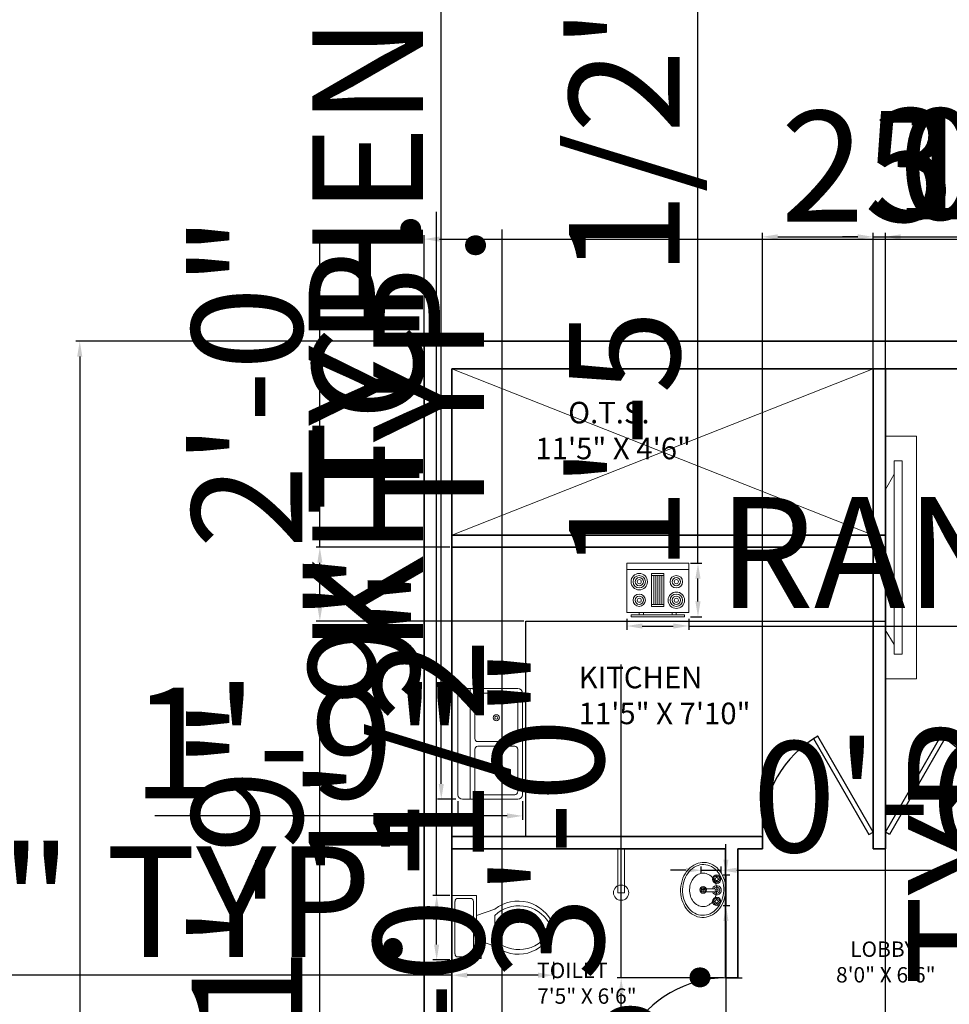
# Model space of a CAD drawing. Units: inches. Extents: x 2901 to 21549, y 2042 to 3828.
# Tile 4 of 10: x 3202 to 3505, y 3259 to 3579. Entities that reach past the tile are written whole.
import ezdxf

# ---------------------------------------------------------------- set-up
doc = ezdxf.new("R2010")
doc.units = ezdxf.units.IN
doc.layers.get('Defpoints').update_dxf_attribs({"color": 1})
for name, color, linetype, lineweight in [('A-ANNO-DIMS', 2, 'Continuous', 18), ('A-AREA-IDEN', 7, 'Continuous', 18), ('A-DOOR', 3, 'Continuous', 25), ('A-EQPM', 8, 'Continuous', 18), ('A-FLOR-CASE', 8, 'Continuous', 25), ('A-FLOR-FIXT', 9, 'Continuous', 18), ('A-ROOF-OPEN', 8, 'Continuous', 13), ('A-WALL', 7, 'Continuous', 35)]:
    doc.layers.add(name, color=color, linetype=linetype, lineweight=lineweight)
doc.styles.get("Standard").update_dxf_attribs({"font": 'arial.ttf'})
doc.dimstyles.new('ISO-25', dxfattribs={"dimtxt": 36, "dimasz": 5, "dimexe": 1.25, "dimexo": 0.625, "dimtad": 1, "dimdec": 0, "dimlunit": 3, "dimtxsty": 'Standard', "dimcen": 2.5, "dimadec": 0, "dimazin": 0, "dimtfac": 1, "dimtdec": 0, "dimtmove": 0, "dimatfit": 3, "dimfxl": 1, "dimarcsym": 0})

# ---------------------------------------------------------------- blocks, each defined once
blk = doc.blocks.new('*U21')
for p, q in [((0, 0), (0, -6)), ((40, 0), (40, -6))]:
    blk.add_line(p, q)
blk.add_lwpolyline([(0, 0), (20, 34.64), (21.52, 33.77), (1.52, -0.88)], close=True)
blk.add_arc((0, 0), 40, 0, 60)
blk = doc.blocks.new('*U22')
for p, q in [((-40, 0), (-40, 6)), ((0, 0), (0, 6))]:
    blk.add_line(p, q)
blk.add_lwpolyline([(0, 0), (-20, -34.64), (-21.52, -33.77), (-1.52, 0.87)], close=True)
blk.add_arc((0, 0), 40, 180, 240)
blk = doc.blocks.new('*U20')
for p, q in [((0, 0), (0, -6)), ((-40, 0), (-40, -6))]:
    blk.add_line(p, q)
blk.add_lwpolyline([(0, 0), (-20, 34.64), (-21.52, 33.77), (-1.52, -0.88)], close=True)
blk.add_arc((0, 0), 40, 120, 180)
blk = doc.blocks.new('Sink - Oval top')
for p, q in [((-1, 0), (1, 0)), ((0, 1), (0, -1))]:
    blk.add_line(p, q)
for points in [[(-12.23, 0.39, 0.117634), (-11.46, -3.36, 0.104469), (-8.88, -6.8, 0.090016), (-5.08, -9.07, 0.08192), (-0.32, -10.02, 0.08192), (4.49, -9.38, 0.090016), (8.42, -7.36, 0.104469), (11.22, -4.09, 0.117634), (12.23, -0.39, 0.117634), (11.46, 3.36, 0.104469), (8.88, 6.8, 0.090016), (5.08, 9.07, 0.08192), (0.32, 10.02, 0.08192), (-4.49, 9.38, 0.090016), (-8.42, 7.36, 0.104469), (-11.22, 4.09, 0.117634)], [(-11.29, 0.16, 0.118622), (-10.52, -3.25, 0.104678), (-8.07, -6.36, 0.089562), (-4.54, -8.37, 0.081185), (-0.13, -9.15, 0.081185), (4.3, -8.49, 0.089562), (7.89, -6.58, 0.104678), (10.42, -3.55, 0.118622), (11.29, -0.16, 0.118622), (10.52, 3.25, 0.104678), (8.07, 6.36, 0.089562), (4.54, 8.37, 0.081185), (0.13, 9.15, 0.081185), (-4.3, 8.49, 0.089562), (-7.89, 6.58, 0.104678), (-10.42, 3.55, 0.118622)], [(-7.42, 0.08, 0.118283), (-6.91, -2.17, 0.104607), (-5.29, -4.21, 0.089718), (-2.97, -5.53, 0.081436), (-0.07, -6.04, 0.081436), (2.84, -5.59, 0.089718), (5.2, -4.33, 0.104607), (6.86, -2.32, 0.118283), (7.42, -0.08, 0.118283), (6.91, 2.17, 0.104607), (5.29, 4.21, 0.089718), (2.97, 5.53, 0.081436), (0.07, 6.04, 0.081436), (-2.84, 5.59, 0.089718), (-5.2, 4.33, 0.104607), (-6.86, 2.32, 0.118283)]]:
    blk.add_lwpolyline(points, format="xyb", close=True)
for radius in [1.5, 1]:
    blk.add_circle((0, 0), radius)
blk = doc.blocks.new('Faucet - Bathroom top')
for p, q in [((-4.107, 0.125), (-4.375, 0.125)), ((-3.75, 0.4788), (-3.75, 0.75)), ((-3.5, 0.482), (-3.5, 0.75)), ((-3.1461, 0.125), (-2.875, 0.125)), ((3.143, 0.125), (2.875, 0.125)), ((3.5, 0.4788), (3.5, 0.75)), ((3.75, 0.482), (3.75, 0.75)), ((4.1039, 0.125), (4.375, 0.125)), ((-4.1039, -0.125), (-4.375, -0.125)), ((-3.75, -0.4821), (-3.75, -0.75)), ((-3.5, -0.4789), (-3.5, -0.75)), ((-3.143, -0.125), (-2.875, -0.125)), ((-0.5, -0.8639), (-0.5, -4.5)), ((0.5, -4.5), (0.5, -0.8631)), ((3.1461, -0.125), (2.875, -0.125)), ((3.5, -0.4821), (3.5, -0.75)), ((3.75, -0.4789), (3.75, -0.75)), ((4.107, -0.125), (4.375, -0.125))]:
    blk.add_line(p, q)
for centre, radius in [((-3.625, 0), 1.375), ((-4.625, 0), 0.2795), ((-3.625, 0), 0.5), ((-3.625, 1), 0.2795), ((-2.625, 0), 0.2795), ((0, 0), 0.5), ((3.625, 0), 1.375), ((2.625, 0), 0.2795), ((3.625, 0), 0.5), ((3.625, 1), 0.2795), ((4.625, 0), 0.2795), ((-3.625, -1), 0.2795), ((3.625, -1), 0.2795)]:
    blk.add_circle(centre, radius)
for centre, radius, start, end in [((-3.625, 0), 1, 105.2407, 164.2093), ((-3.625, 0), 1, 16.44125, 74.07887), ((0, 0), 1.5, 289.6514, 250.3603), ((0, 0), 1, 300.3431, 239.7554), ((3.625, 0), 1, 106.12, 164.0884), ((3.625, 0), 1, 16.23422, 73.90469), ((-3.625, 0), 1, 196.2342, 253.9047), ((-3.625, 0), 1, 286.12, 344.0884), ((3.625, 0), 1, 196.4413, 254.0789), ((3.625, 0), 1, 285.2407, 344.2093), ((0, -4.5), 0.5, 180, 0)]:
    blk.add_arc(centre, radius, start, end)
blk = doc.blocks.new('Range-Oven - 30 in top')
for p, q in [((0, -3), (30, -3)), ((12, -6), (18, -6)), ((13, -20), (13, -6)), ((14, -6), (14, -20)), ((15, -20), (15, -6)), ((16, -6), (16, -20)), ((17, -20), (17, -6)), ((18, -20), (12, -20)), ((6, -24), (6, -25)), ((8, -25), (8, -24)), ((22, -25), (22, -24)), ((24, -24), (24, -25))]:
    blk.add_line(p, q)
for points in [[(0, -24), (0, 0), (30, 0), (30, -24)], [(12, -21), (12, -5), (18, -5), (18, -21)], [(2, -26), (2, -25), (28, -25), (28, -26)]]:
    blk.add_lwpolyline(points, close=True)
for centre, radius in [((6, -9), 4), ((6, -9), 3), ((6, -9), 2), ((6, -9), 1), ((24, -9), 3), ((24, -9), 2), ((24, -9), 1), ((24, -18), 4), ((6, -18), 3), ((6, -18), 2), ((6, -18), 1), ((24, -18), 3), ((24, -18), 2), ((24, -18), 1)]:
    blk.add_circle(centre, radius)
blk = doc.blocks.new('Sink-double - 36 in top')
for p, q in [((-18, -4), (18, -4)), ((-0.75, -18.5), (-0.75, -6.5)), ((0.75, -6.5), (0.75, -18.5))]:
    blk.add_line(p, q)
for points in [[(-16.5, 0), (16.5, 0)], [(-18, -19.5), (-18, -1.5)], [(18, -1.5), (18, -19.5)], [(-15.5, -5.5), (-1.75, -5.5)], [(1.75, -5.5), (15.5, -5.5)], [(-16.5, -18.5), (-16.5, -6.5)], [(16.5, -6.5), (16.5, -18.5)], [(16.5, -21), (-16.5, -21)], [(-1.75, -19.5), (-15.5, -19.5)], [(15.5, -19.5), (1.75, -19.5)]]:
    blk.add_lwpolyline(points)
for centre, radius in [((-8.5, -12.5), 1), ((-8.5, -12.5), 0.5), ((8.5, -12.5), 1), ((8.5, -12.5), 0.5)]:
    blk.add_circle(centre, radius)
for centre, radius, start, end in [((-16.5, -1.5), 1.5, 90, 180), ((16.5, -1.5), 1.5, 0, 90), ((-15.5, -6.5), 1, 90, 180), ((-1.75, -6.5), 1, 0, 90), ((1.75, -6.5), 1, 90, 180), ((15.5, -6.5), 1, 0, 90), ((-15.5, -18.5), 1, 180, 270), ((-1.75, -18.5), 1, 270, 0), ((1.75, -18.5), 1, 180, 270), ((15.5, -18.5), 1, 270, 0), ((-16.5, -19.5), 1.5, 180, 270), ((16.5, -19.5), 1.5, 270, 0)]:
    blk.add_arc(centre, radius, start, end)
blk = doc.blocks.new('Toilet - top')
for p, q in [((9.5, -6), (9.5, -2)), ((-10, -8.5), (-8, -8.5)), ((-10, -9.5), (-10, -8.5)), ((-7, -9.5), (-10, -9.5)), ((-8, -8.5), (-8, -8)), ((-7, -8), (-7, -9.5)), ((-4, -8), (-6, -14)), ((4, -8), (6, -14)), ((4, -14), (-4, -14))]:
    blk.add_line(p, q)
blk.add_lwpolyline([(10.5, -8), (10.5, 0), (-10.5, 0), (-10.5, -8)], close=True)
for points in [[(-9.5, -2), (-9.5, -6)], [(8.5, -1), (-8.5, -1)], [(-8.5, -7), (8.5, -7)]]:
    blk.add_lwpolyline(points)
for centre, radius, start, end in [((-8.62, -1.88), 0.884, 81.8699, 188.1301), ((8.62, -1.88), 0.884, 351.8699, 98.1301), ((-8.62, -6.12), 0.884, 171.8699, 278.1301), ((8.62, -6.12), 0.884, 261.8699, 8.1301), ((3.52, -21.58), 12.17, 141.4691, 247.9714), ((4.2, -21.82), 11.33, 136.3677, 238.9468), ((-3.52, -21.58), 12.17, 292.0284, 38.5307), ((-4.2, -21.82), 11.33, 301.053, 43.6321), ((0, -27.88), 4, 245.7318, 294.2682), ((0, -29), 4, 254.8605, 285.1395)]:
    blk.add_arc(centre, radius, start, end)
blk = doc.blocks.new('*D30')
at = {"layer": 'A-ANNO-DIMS', "color": 0, "lineweight": -2, "transparency": 16777216}
for p, q in [((3334.07, 3475.1), (3334.07, 3508.95)), ((3634.07, 3475.1), (3634.07, 3508.95)), ((3339.07, 3507.7), (3629.07, 3507.7))]:
    blk.add_line(p, q, dxfattribs=at)
at = {"layer": 'A-ANNO-DIMS', "color": 0, "transparency": 16777216}
for points in [[(3339.07, 3508.53), (3339.07, 3506.87), (3334.07, 3507.7)], [(3629.07, 3508.53), (3629.07, 3506.87), (3634.07, 3507.7)]]:
    blk.add_solid(points, dxfattribs=at)
at = {"layer": 'Defpoints', "color": 0, "transparency": 16777216}
for p in [(3634.07, 3507.7), (3334.07, 3474.48), (3634.07, 3474.48)]:
    blk.add_point(p, dxfattribs=at)
at = {"layer": 'A-ANNO-DIMS', "color": 0, "transparency": 16777216, "insert": (3484.07, 3526.7), "char_height": 36, "attachment_point": 5}
blk.add_mtext("25'", dxfattribs=at)
blk = doc.blocks.new('*D31')
at = {"layer": 'A-ANNO-DIMS', "color": 0, "lineweight": -2, "transparency": 16777216}
for p, q in [((3333.44, 3474.48), (3220.78, 3474.48)), ((3222.03, 3469.48), (3222.03, 2879.48)), ((3333.44, 2874.48), (3220.78, 2874.48))]:
    blk.add_line(p, q, dxfattribs=at)
at = {"layer": 'A-ANNO-DIMS', "color": 0, "transparency": 16777216}
for points in [[(3221.19, 3469.48), (3222.86, 3469.48), (3222.03, 3474.48)], [(3221.19, 2879.48), (3222.86, 2879.48), (3222.03, 2874.48)]]:
    blk.add_solid(points, dxfattribs=at)
at = {"layer": 'Defpoints', "color": 0, "transparency": 16777216}
for p in [(3334.07, 3474.48), (3222.03, 2874.48), (3334.07, 2874.48)]:
    blk.add_point(p, dxfattribs=at)
at = {"layer": 'A-ANNO-DIMS', "color": 0, "transparency": 16777216, "insert": (3203.02, 3174.48), "char_height": 36, "attachment_point": 5, "rotation": 90}
blk.add_mtext("50'", dxfattribs=at)
blk = doc.blocks.new('BEDROOM-MEDIA-UNIT')
for p, q in [((2.89, 66.49), (0, 61.37)), ((0, 15.88), (2.89, 11.11))]:
    blk.add_line(p, q)
for points in [[(0.06, 78.84), (10.18, 78.84), (10.18, 0), (0.06, 0)], [(2.89, 70.84), (5.46, 70.84), (5.46, 8), (2.89, 8)]]:
    blk.add_lwpolyline(points, close=True)
blk = doc.blocks.new('*D38')
at = {"layer": 'A-ANNO-DIMS', "color": 0, "lineweight": -2, "transparency": 16777216}
for p, q in [((3343.07, 3191.34), (3343.07, 3188.58)), ((3348.07, 3189.83), (3352.29, 3189.83)), ((3357.29, 3191.34), (3357.29, 3188.58)), ((3357.29, 3189.83), (3922.11, 3189.83))]:
    blk.add_line(p, q, dxfattribs=at)
at = {"layer": 'A-ANNO-DIMS', "color": 0, "transparency": 16777216}
for points in [[(3348.07, 3190.67), (3348.07, 3189), (3343.07, 3189.83)], [(3352.29, 3190.67), (3352.29, 3189), (3357.29, 3189.83)]]:
    blk.add_solid(points, dxfattribs=at)
at = {"layer": 'Defpoints', "color": 0, "transparency": 16777216}
for p in [(3343.07, 3191.97), (3357.29, 3191.97), (3357.29, 3189.83)]:
    blk.add_point(p, dxfattribs=at)
at = {"layer": 'A-ANNO-DIMS', "color": 0, "transparency": 16777216, "insert": (3642.2, 3209.07), "char_height": 36, "attachment_point": 5}
blk.add_mtext('NIGHTSTAND 1\'-2" TYP.', dxfattribs=at)
blk = doc.blocks.new('*D39')
at = {"layer": 'A-ANNO-DIMS', "color": 0, "lineweight": -2, "transparency": 16777216}
for p, q in [((3359.43, 3204.67), (3359.43, 3510.85)), ((3357.92, 3204.67), (3360.68, 3204.67)), ((3359.43, 3196.97), (3359.43, 3199.67)), ((3357.92, 3191.97), (3360.68, 3191.97))]:
    blk.add_line(p, q, dxfattribs=at)
at = {"layer": 'A-ANNO-DIMS', "color": 0, "transparency": 16777216}
for points in [[(3358.59, 3199.67), (3360.26, 3199.67), (3359.43, 3204.67)], [(3358.59, 3196.97), (3360.26, 3196.97), (3359.43, 3191.97)]]:
    blk.add_solid(points, dxfattribs=at)
at = {"layer": 'Defpoints', "color": 0, "transparency": 16777216}
for p in [(3357.29, 3204.67), (3359.43, 3204.67), (3357.29, 3191.97)]:
    blk.add_point(p, dxfattribs=at)
at = {"layer": 'A-ANNO-DIMS', "color": 0, "transparency": 16777216, "insert": (3340.19, 3360.26), "char_height": 36, "attachment_point": 5, "rotation": 90}
blk.add_mtext('1\'-0 1/2" TYP.', dxfattribs=at)
blk = doc.blocks.new('*D40')
at = {"layer": 'A-ANNO-DIMS', "color": 0, "lineweight": -2, "transparency": 16777216}
for p, q in [((3343.07, 3272.69), (3343.07, 3267.11)), ((3376.12, 3272.69), (3376.12, 3267.11)), ((3343.07, 3268.36), (3018.15, 3268.36)), ((3371.12, 3268.36), (3348.07, 3268.36))]:
    blk.add_line(p, q, dxfattribs=at)
at = {"layer": 'A-ANNO-DIMS', "color": 0, "transparency": 16777216}
for points in [[(3348.07, 3269.19), (3348.07, 3267.52), (3343.07, 3268.36)], [(3371.12, 3269.19), (3371.12, 3267.52), (3376.12, 3268.36)]]:
    blk.add_solid(points, dxfattribs=at)
at = {"layer": 'Defpoints', "color": 0, "transparency": 16777216}
for p in [(3343.07, 3273.32), (3376.12, 3273.32), (3343.07, 3268.36)]:
    blk.add_point(p, dxfattribs=at)
at = {"layer": 'A-ANNO-DIMS', "color": 0, "transparency": 16777216, "insert": (3178.11, 3287.6), "char_height": 36, "attachment_point": 5}
blk.add_mtext('WC 2\'-9" TYP.', dxfattribs=at)
blk = doc.blocks.new('*D41')
at = {"layer": 'A-ANNO-DIMS', "color": 0, "lineweight": -2, "transparency": 16777216}
for p, q in [((3338.11, 3294.32), (3338.11, 3516.61)), ((3342.44, 3294.32), (3336.86, 3294.32)), ((3338.11, 3278.32), (3338.11, 3289.32)), ((3342.44, 3273.32), (3336.86, 3273.32))]:
    blk.add_line(p, q, dxfattribs=at)
at = {"layer": 'A-ANNO-DIMS', "color": 0, "transparency": 16777216}
for points in [[(3337.28, 3289.32), (3338.95, 3289.32), (3338.11, 3294.32)], [(3337.28, 3278.32), (3338.95, 3278.32), (3338.11, 3273.32)]]:
    blk.add_solid(points, dxfattribs=at)
at = {"layer": 'Defpoints', "color": 0, "transparency": 16777216}
for p in [(3338.11, 3294.32), (3343.07, 3294.32), (3343.07, 3273.32)]:
    blk.add_point(p, dxfattribs=at)
at = {"layer": 'A-ANNO-DIMS', "color": 0, "transparency": 16777216, "insert": (3319.11, 3407.96), "char_height": 36, "attachment_point": 5, "rotation": 90}
blk.add_mtext('1\'-9" TYP.', dxfattribs=at)
blk = doc.blocks.new('*D42')
at = {"layer": 'A-ANNO-DIMS', "color": 0, "lineweight": -2, "transparency": 16777216}
for p, q in [((3533.42, 3266.44), (3528.38, 3599.53)), ((3535.49, 3266.47), (3532.17, 3266.42)), ((3533.62, 3253.49), (3533.5, 3261.44)), ((3535.76, 3248.52), (3532.44, 3248.47))]:
    blk.add_line(p, q, dxfattribs=at)
at = {"layer": 'A-ANNO-DIMS', "color": 0, "transparency": 16777216}
for points in [[(3534.33, 3261.45), (3532.66, 3261.43), (3533.42, 3266.44)], [(3534.45, 3253.5), (3532.78, 3253.48), (3533.69, 3248.49)]]:
    blk.add_solid(points, dxfattribs=at)
at = {"layer": 'Defpoints', "color": 0, "transparency": 16777216}
for p in [(3533.42, 3266.44), (3536.11, 3266.48), (3536.39, 3248.53)]:
    blk.add_point(p, dxfattribs=at)
at = {"layer": 'A-ANNO-DIMS', "color": 0, "transparency": 16777216, "insert": (3549.86, 3435.77), "char_height": 36, "attachment_point": 5, "rotation": 270.8679}
blk.add_mtext('LAV 1\'-6" TYP.', dxfattribs=at)
blk = doc.blocks.new('*D44')
at = {"layer": 'A-ANNO-DIMS', "color": 0, "lineweight": -2, "transparency": 16777216}
for p, q in [((3432.19, 3305.97), (3432.19, 3310.97)), ((3431.32, 3300.97), (3433.44, 3300.97)), ((3432.19, 3300.97), (3432.19, 3290.97)), ((3431.32, 3290.97), (3433.44, 3290.97)), ((3432.19, 3285.97), (3432.19, 2919.63))]:
    blk.add_line(p, q, dxfattribs=at)
at = {"layer": 'A-ANNO-DIMS', "color": 0, "transparency": 16777216}
for points in [[(3431.36, 3305.97), (3433.02, 3305.97), (3432.19, 3300.97)], [(3431.36, 3285.97), (3433.02, 3285.97), (3432.19, 3290.97)]]:
    blk.add_solid(points, dxfattribs=at)
at = {"layer": 'Defpoints', "color": 0, "transparency": 16777216}
for p in [(3430.69, 3300.97), (3430.69, 3290.97), (3432.19, 3290.97)]:
    blk.add_point(p, dxfattribs=at)
at = {"layer": 'A-ANNO-DIMS', "color": 0, "transparency": 16777216, "insert": (3413.18, 3100.3), "char_height": 36, "attachment_point": 5, "rotation": 90}
blk.add_mtext('TAP 0\'-10" TYP.', dxfattribs=at)
blk = doc.blocks.new('*D45')
at = {"layer": 'A-ANNO-DIMS', "color": 0, "lineweight": -2, "transparency": 16777216}
for p, q in [((3419.19, 3302.47), (3414.19, 3302.47)), ((3424.19, 3301.6), (3424.19, 3303.72)), ((3424.19, 3302.47), (3430.69, 3302.47)), ((3430.69, 3301.6), (3430.69, 3303.72)), ((3435.69, 3302.47), (3745.26, 3302.47))]:
    blk.add_line(p, q, dxfattribs=at)
at = {"layer": 'A-ANNO-DIMS', "color": 0, "transparency": 16777216}
for points in [[(3419.19, 3303.31), (3419.19, 3301.64), (3424.19, 3302.47)], [(3435.69, 3303.31), (3435.69, 3301.64), (3430.69, 3302.47)]]:
    blk.add_solid(points, dxfattribs=at)
at = {"layer": 'Defpoints', "color": 0, "transparency": 16777216}
for p in [(3424.19, 3300.97), (3430.69, 3302.47), (3430.69, 3300.97)]:
    blk.add_point(p, dxfattribs=at)
at = {"layer": 'A-ANNO-DIMS', "color": 0, "transparency": 16777216, "insert": (3592.98, 3321.71), "char_height": 36, "attachment_point": 5}
blk.add_mtext('0\'-6 1/2" TYP.', dxfattribs=at)
blk = doc.blocks.new('*D47')
at = {"layer": 'A-ANNO-DIMS', "color": 0, "lineweight": -2, "transparency": 16777216}
for p, q in [((3544.44, 3430.67), (3531.82, 3430.67)), ((3533.07, 3425.67), (3533.07, 3375.67)), ((3544.44, 3370.67), (3531.82, 3370.67)), ((3533.07, 3370.67), (3533.07, 3144.99))]:
    blk.add_line(p, q, dxfattribs=at)
at = {"layer": 'A-ANNO-DIMS', "color": 0, "transparency": 16777216}
for points in [[(3532.24, 3425.67), (3533.9, 3425.67), (3533.07, 3430.67)], [(3532.24, 3375.67), (3533.9, 3375.67), (3533.07, 3370.67)]]:
    blk.add_solid(points, dxfattribs=at)
at = {"layer": 'Defpoints', "color": 0, "transparency": 16777216}
for p in [(3545.07, 3430.67), (3533.07, 3370.67), (3545.07, 3370.67)]:
    blk.add_point(p, dxfattribs=at)
at = {"layer": 'A-ANNO-DIMS', "color": 0, "transparency": 16777216, "insert": (3514.06, 3255.33), "char_height": 36, "attachment_point": 5, "rotation": 90}
blk.add_mtext('5\'-0" TYP.', dxfattribs=at)
blk = doc.blocks.new('*D53')
at = {"layer": 'A-ANNO-DIMS', "color": 0, "lineweight": -2, "transparency": 16777216}
for p, q in [((3464.89, 3209.18), (3211.23, 3209.18)), ((3469.89, 3197.98), (3469.89, 3210.43)), ((3480.07, 3209.18), (3469.89, 3209.18)), ((3480.07, 3197.98), (3480.07, 3210.43)), ((3485.07, 3209.18), (3490.07, 3209.18))]:
    blk.add_line(p, q, dxfattribs=at)
at = {"layer": 'A-ANNO-DIMS', "color": 0, "transparency": 16777216}
for points in [[(3464.89, 3210.01), (3464.89, 3208.34), (3469.89, 3209.18)], [(3485.07, 3210.01), (3485.07, 3208.34), (3480.07, 3209.18)]]:
    blk.add_solid(points, dxfattribs=at)
at = {"layer": 'Defpoints', "color": 0, "transparency": 16777216}
for p in [(3469.89, 3209.18), (3469.89, 3197.35), (3480.07, 3197.35)]:
    blk.add_point(p, dxfattribs=at)
at = {"layer": 'A-ANNO-DIMS', "color": 0, "transparency": 16777216, "insert": (3335.56, 3228.18), "char_height": 36, "attachment_point": 5}
blk.add_mtext('0\'-10" TYP.', dxfattribs=at)
blk = doc.blocks.new('*D58')
at = {"layer": 'A-ANNO-DIMS', "color": 0, "lineweight": -2, "transparency": 16777216}
for p, q in [((3399.98, 3384.28), (3399.98, 3380.64)), ((3420.08, 3384.28), (3420.08, 3380.64)), ((3404.98, 3381.89), (3415.08, 3381.89)), ((3420.08, 3381.89), (3712.98, 3381.89))]:
    blk.add_line(p, q, dxfattribs=at)
at = {"layer": 'A-ANNO-DIMS', "color": 0, "transparency": 16777216}
for points in [[(3404.98, 3382.72), (3404.98, 3381.06), (3399.98, 3381.89)], [(3415.08, 3382.72), (3415.08, 3381.06), (3420.08, 3381.89)]]:
    blk.add_solid(points, dxfattribs=at)
at = {"layer": 'Defpoints', "color": 0, "transparency": 16777216}
for p in [(3399.98, 3384.91), (3420.08, 3384.91), (3420.08, 3381.89)]:
    blk.add_point(p, dxfattribs=at)
at = {"layer": 'A-ANNO-DIMS', "color": 0, "transparency": 16777216, "insert": (3569.03, 3401.13), "char_height": 36, "attachment_point": 5}
blk.add_mtext('RANGE 1\'-8"', dxfattribs=at)
blk = doc.blocks.new('*D59')
at = {"layer": 'A-ANNO-DIMS', "color": 0, "lineweight": -2, "transparency": 16777216}
for p, q in [((3423.1, 3402.33), (3423.1, 3584.77)), ((3420.71, 3402.33), (3424.35, 3402.33)), ((3423.1, 3389.91), (3423.1, 3397.33)), ((3420.71, 3384.91), (3424.35, 3384.91))]:
    blk.add_line(p, q, dxfattribs=at)
at = {"layer": 'A-ANNO-DIMS', "color": 0, "transparency": 16777216}
for points in [[(3422.26, 3397.33), (3423.93, 3397.33), (3423.1, 3402.33)], [(3422.26, 3389.91), (3423.93, 3389.91), (3423.1, 3384.91)]]:
    blk.add_solid(points, dxfattribs=at)
at = {"layer": 'Defpoints', "color": 0, "transparency": 16777216}
for p in [(3420.08, 3402.33), (3423.1, 3402.33), (3420.08, 3384.91)]:
    blk.add_point(p, dxfattribs=at)
at = {"layer": 'A-ANNO-DIMS', "color": 0, "transparency": 16777216, "insert": (3403.86, 3496.05), "char_height": 36, "attachment_point": 5, "rotation": 90}
blk.add_mtext('1\'-5 1/2"', dxfattribs=at)
blk = doc.blocks.new('*D60')
at = {"layer": 'A-ANNO-DIMS', "color": 0, "lineweight": -2, "transparency": 16777216}
for p, q in [((3339.61, 3361.55), (3339.61, 3827.97)), ((3344.38, 3361.55), (3338.36, 3361.55)), ((3339.61, 3330.55), (3339.61, 3356.55)), ((3344.38, 3325.55), (3338.36, 3325.55))]:
    blk.add_line(p, q, dxfattribs=at)
at = {"layer": 'A-ANNO-DIMS', "color": 0, "transparency": 16777216}
for points in [[(3338.78, 3356.55), (3340.44, 3356.55), (3339.61, 3361.55)], [(3338.78, 3330.55), (3340.44, 3330.55), (3339.61, 3325.55)]]:
    blk.add_solid(points, dxfattribs=at)
at = {"layer": 'Defpoints', "color": 0, "transparency": 16777216}
for p in [(3339.61, 3361.55), (3345.01, 3361.55), (3345.01, 3325.55)]:
    blk.add_point(p, dxfattribs=at)
at = {"layer": 'A-ANNO-DIMS', "color": 0, "transparency": 16777216, "insert": (3320.36, 3597.26), "char_height": 36, "attachment_point": 5, "rotation": 90}
blk.add_mtext('KITCHEN SINK 3\'-0"', dxfattribs=at)
blk = doc.blocks.new('*D61')
at = {"layer": 'A-ANNO-DIMS', "color": 0, "lineweight": -2, "transparency": 16777216}
for p, q in [((3345.01, 3324.93), (3345.01, 3318.9)), ((3366.01, 3324.93), (3366.01, 3318.9)), ((3345.01, 3320.15), (3246.45, 3320.15)), ((3361.01, 3320.15), (3350.01, 3320.15))]:
    blk.add_line(p, q, dxfattribs=at)
at = {"layer": 'A-ANNO-DIMS', "color": 0, "transparency": 16777216}
for points in [[(3350.01, 3320.99), (3350.01, 3319.32), (3345.01, 3320.15)], [(3361.01, 3320.99), (3361.01, 3319.32), (3366.01, 3320.15)]]:
    blk.add_solid(points, dxfattribs=at)
at = {"layer": 'Defpoints', "color": 0, "transparency": 16777216}
for p in [(3345.01, 3325.55), (3366.01, 3325.55), (3345.01, 3320.15)]:
    blk.add_point(p, dxfattribs=at)
at = {"layer": 'A-ANNO-DIMS', "color": 0, "transparency": 16777216, "insert": (3293.23, 3339.16), "char_height": 36, "attachment_point": 5}
blk.add_mtext('1\'-9"', dxfattribs=at)
blk = doc.blocks.new('*D67')
at = {"layer": 'A-ANNO-DIMS', "color": 0, "lineweight": -2, "transparency": 16777216}
for p, q in [((3484.07, 3013.1), (3484.07, 3509.68)), ((3625.07, 3228.1), (3625.07, 3509.68)), ((3489.07, 3508.43), (3620.07, 3508.43))]:
    blk.add_line(p, q, dxfattribs=at)
at = {"layer": 'A-ANNO-DIMS', "color": 0, "transparency": 16777216}
for points in [[(3489.07, 3509.26), (3489.07, 3507.59), (3484.07, 3508.43)], [(3620.07, 3509.26), (3620.07, 3507.59), (3625.07, 3508.43)]]:
    blk.add_solid(points, dxfattribs=at)
at = {"layer": 'Defpoints', "color": 0, "transparency": 16777216}
for p in [(3625.07, 3508.43), (3625.07, 3227.48), (3484.07, 3012.48)]:
    blk.add_point(p, dxfattribs=at)
at = {"layer": 'A-ANNO-DIMS', "color": 0, "transparency": 16777216, "insert": (3554.57, 3527.43), "char_height": 36, "attachment_point": 5}
blk.add_mtext('11\'-9"', dxfattribs=at)
blk = doc.blocks.new('*D77')
at = {"layer": 'A-ANNO-DIMS', "color": 0, "lineweight": -2, "transparency": 16777216}
for p, q in [((3480.07, 3310.1), (3480.07, 3509.68)), ((3484.07, 3310.1), (3484.07, 3509.68)), ((3475.07, 3508.43), (3470.07, 3508.43)), ((3480.07, 3508.43), (3484.07, 3508.43)), ((3489.07, 3508.43), (3591.02, 3508.43))]:
    blk.add_line(p, q, dxfattribs=at)
at = {"layer": 'A-ANNO-DIMS', "color": 0, "transparency": 16777216}
for points in [[(3475.07, 3509.26), (3475.07, 3507.59), (3480.07, 3508.43)], [(3489.07, 3509.26), (3489.07, 3507.59), (3484.07, 3508.43)]]:
    blk.add_solid(points, dxfattribs=at)
at = {"layer": 'Defpoints', "color": 0, "transparency": 16777216}
for p in [(3484.07, 3508.43), (3480.07, 3309.48), (3484.07, 3309.48)]:
    blk.add_point(p, dxfattribs=at)
at = {"layer": 'A-ANNO-DIMS', "color": 0, "transparency": 16777216, "insert": (3542.54, 3527.43), "char_height": 36, "attachment_point": 5}
blk.add_mtext('0\'-4"', dxfattribs=at)
blk = doc.blocks.new('*D79')
at = {"layer": 'A-ANNO-DIMS', "color": 0, "lineweight": -2, "transparency": 16777216}
for p, q in [((3300.12, 3252.55), (3300.12, 3351.11)), ((3342.44, 3252.55), (3298.87, 3252.55)), ((3300.12, 3236.48), (3300.12, 3247.55)), ((3342.44, 3231.48), (3298.87, 3231.48))]:
    blk.add_line(p, q, dxfattribs=at)
at = {"layer": 'A-ANNO-DIMS', "color": 0, "transparency": 16777216}
for points in [[(3299.29, 3247.55), (3300.95, 3247.55), (3300.12, 3252.55)], [(3299.29, 3236.48), (3300.95, 3236.48), (3300.12, 3231.48)]]:
    blk.add_solid(points, dxfattribs=at)
at = {"layer": 'Defpoints', "color": 0, "transparency": 16777216}
for p in [(3300.12, 3252.55), (3343.07, 3252.55), (3343.07, 3231.48)]:
    blk.add_point(p, dxfattribs=at)
at = {"layer": 'A-ANNO-DIMS', "color": 0, "transparency": 16777216, "insert": (3281.11, 3304.33), "char_height": 36, "attachment_point": 5, "rotation": 90}
blk.add_mtext('1\'-9"', dxfattribs=at)
blk = doc.blocks.new('*D80')
at = {"layer": 'A-ANNO-DIMS', "color": 0, "lineweight": -2, "transparency": 16777216}
for p, q in [((3300.12, 3407.48), (3300.12, 3510.04)), ((3342.44, 3407.48), (3298.87, 3407.48)), ((3300.12, 3388.48), (3300.12, 3402.48)), ((3366.44, 3383.48), (3298.87, 3383.48))]:
    blk.add_line(p, q, dxfattribs=at)
at = {"layer": 'A-ANNO-DIMS', "color": 0, "transparency": 16777216}
for points in [[(3299.29, 3402.48), (3300.95, 3402.48), (3300.12, 3407.48)], [(3299.29, 3388.48), (3300.95, 3388.48), (3300.12, 3383.48)]]:
    blk.add_solid(points, dxfattribs=at)
at = {"layer": 'Defpoints', "color": 0, "transparency": 16777216}
for p in [(3300.12, 3407.48), (3343.07, 3407.48), (3367.07, 3383.48)]:
    blk.add_point(p, dxfattribs=at)
at = {"layer": 'A-ANNO-DIMS', "color": 0, "transparency": 16777216, "insert": (3281.11, 3461.26), "char_height": 36, "attachment_point": 5, "rotation": 90}
blk.add_mtext('2\'-0"', dxfattribs=at)
blk = doc.blocks.new('*D81')
at = {"layer": 'A-ANNO-DIMS', "color": 0, "lineweight": -2, "transparency": 16777216}
for p, q in [((3444.07, 3314.1), (3444.07, 3509.68)), ((3480.07, 3314.1), (3480.07, 3509.68)), ((3449.07, 3508.43), (3475.07, 3508.43)), ((3480.07, 3508.43), (3581.99, 3508.43))]:
    blk.add_line(p, q, dxfattribs=at)
at = {"layer": 'A-ANNO-DIMS', "color": 0, "transparency": 16777216}
for points in [[(3449.07, 3509.26), (3449.07, 3507.59), (3444.07, 3508.43)], [(3475.07, 3509.26), (3475.07, 3507.59), (3480.07, 3508.43)]]:
    blk.add_solid(points, dxfattribs=at)
at = {"layer": 'Defpoints', "color": 0, "transparency": 16777216}
for p in [(3480.07, 3508.43), (3444.07, 3313.48), (3480.07, 3313.48)]:
    blk.add_point(p, dxfattribs=at)
at = {"layer": 'A-ANNO-DIMS', "color": 0, "transparency": 16777216, "insert": (3533.53, 3527.45), "char_height": 36, "attachment_point": 5}
blk.add_mtext('3\'-0"', dxfattribs=at)
blk = doc.blocks.new('*D82')
at = {"layer": 'A-ANNO-DIMS', "color": 0, "lineweight": -2, "transparency": 16777216}
for p, q in [((3484.07, 3313.93), (3484.07, 3509.68)), ((3520.07, 3314.1), (3520.07, 3509.68)), ((3489.07, 3508.43), (3515.07, 3508.43)), ((3520.07, 3508.43), (3621.99, 3508.43))]:
    blk.add_line(p, q, dxfattribs=at)
at = {"layer": 'A-ANNO-DIMS', "color": 0, "transparency": 16777216}
for points in [[(3489.07, 3509.26), (3489.07, 3507.59), (3484.07, 3508.43)], [(3515.07, 3509.26), (3515.07, 3507.59), (3520.07, 3508.43)]]:
    blk.add_solid(points, dxfattribs=at)
at = {"layer": 'Defpoints', "color": 0, "transparency": 16777216}
for p in [(3520.07, 3508.43), (3520.07, 3313.48), (3484.07, 3313.3)]:
    blk.add_point(p, dxfattribs=at)
at = {"layer": 'A-ANNO-DIMS', "color": 0, "transparency": 16777216, "insert": (3573.53, 3527.45), "char_height": 36, "attachment_point": 5}
blk.add_mtext('3\'-0"', dxfattribs=at)
blk = doc.blocks.new('*D83')
at = {"layer": 'A-ANNO-DIMS', "color": 0, "lineweight": -2, "transparency": 16777216}
for p, q in [((3398.12, 3267.48), (3398.12, 3369.4)), ((3431.44, 3267.48), (3396.87, 3267.48)), ((3398.12, 3236.48), (3398.12, 3262.48)), ((3431.44, 3231.48), (3396.87, 3231.48))]:
    blk.add_line(p, q, dxfattribs=at)
at = {"layer": 'A-ANNO-DIMS', "color": 0, "transparency": 16777216}
for points in [[(3397.29, 3262.48), (3398.95, 3262.48), (3398.12, 3267.48)], [(3397.29, 3236.48), (3398.95, 3236.48), (3398.12, 3231.48)]]:
    blk.add_solid(points, dxfattribs=at)
at = {"layer": 'Defpoints', "color": 0, "transparency": 16777216}
for p in [(3398.12, 3267.48), (3432.07, 3267.48), (3432.07, 3231.48)]:
    blk.add_point(p, dxfattribs=at)
at = {"layer": 'A-ANNO-DIMS', "color": 0, "transparency": 16777216, "insert": (3379.1, 3320.94), "char_height": 36, "attachment_point": 5, "rotation": 90}
blk.add_mtext('3\'-0"', dxfattribs=at)

msp = doc.modelspace()

# ---------------------------------------------------------------- linework, layer by layer
at = {"layer": 'A-EQPM'}
msp.add_line((3484.07, 3401.04), (3484.07, 3355.55), dxfattribs=at)
at = {"layer": 'A-FLOR-CASE'}
for p, q in [((3367.07, 3383.48), (3484.07, 3383.48)), ((3367.07, 3313.48), (3367.07, 3383.48))]:
    msp.add_line(p, q, dxfattribs=at)
at = {"layer": 'A-FLOR-FIXT'}
for p, q in [((3397.04, 3309.48), (3397.04, 3295.19)), ((3399.16, 3295.19), (3399.16, 3309.48)), ((3397.04, 3295.19), (3399.16, 3295.19))]:
    msp.add_line(p, q, dxfattribs=at)
msp.add_circle((3398.11, 3295.19), 2.49, dxfattribs=at)
at = {"layer": 'A-ROOF-OPEN'}
for p, q in [((3480.07, 3411.48), (3343.07, 3465.48)), ((3343.07, 3411.48), (3480.07, 3465.48))]:
    msp.add_line(p, q, dxfattribs=at)
at = {"layer": 'A-WALL'}
for p, q in [((3343.07, 2883.48), (3343.07, 3465.48)), ((3343.07, 3465.48), (3625.07, 3465.48)), ((3480.07, 3309.48), (3480.07, 3465.48)), ((3484.07, 3309.48), (3484.07, 3465.48)), ((3343.07, 3411.48), (3484.07, 3411.48)), ((3343.07, 3407.48), (3484.07, 3407.48)), ((3343.07, 3313.48), (3444.07, 3313.48)), ((3444.07, 3309.48), (3444.07, 3313.48)), ((3480.07, 3309.48), (3480.07, 3313.48)), ((3343.07, 3309.48), (3432.07, 3309.48)), ((3432.07, 3267.48), (3432.07, 3309.48)), ((3436.07, 3309.48), (3444.07, 3309.48)), ((3436.07, 3267.48), (3436.07, 3309.48)), ((3480.07, 3309.48), (3484.07, 3309.48)), ((3432.07, 3267.48), (3436.07, 3267.48))]:
    msp.add_line(p, q, dxfattribs=at)
msp.add_lwpolyline([(3634.07, 3474.48), (3634.07, 2874.48), (3334.07, 2874.48), (3334.07, 3474.48)], close=True, dxfattribs=at)

# ---------------------------------------------------------------- block references
at = {"layer": 'A-DOOR'}
for name, p, xscale, yscale, zscale in [('*U20', (3480.07, 3314.88), 0.9, 0.9, 0.9), ('*U21', (3484.07, 3314.88), 0.8999999999999834, 0.8999999999999834, 0.8999999999999834)]:
    msp.add_blockref(name, p, dxfattribs=dict(at, xscale=xscale, yscale=yscale, zscale=zscale))
at = {"layer": 'A-DOOR', "xscale": 0.8999999999999889, "yscale": 0.8999999999999889, "zscale": 0.8999999999999889, "rotation": 270.0000000000072}
msp.add_blockref('*U22', (3432.07, 3231.48), dxfattribs=at)
at = {"layer": 'A-EQPM'}
msp.add_blockref('BEDROOM-MEDIA-UNIT', (3484.01, 3364.74), dxfattribs=at)
at = {"layer": 'A-EQPM', "xscale": 0.6699917200151848, "yscale": 0.6699917200151848, "zscale": 0.6699917200151848}
msp.add_blockref('Range-Oven - 30 in top', (3399.98, 3402.33), dxfattribs=at)
at = {"layer": 'A-FLOR-FIXT'}
for name, p, rotation in [('Sink-double - 36 in top', (3345.01, 3343.55), 90), ('Faucet - Bathroom top', (3429.19, 3295.97), 270), ('Toilet - top', (3343.07, 3283.82), 89.99999999999999)]:
    msp.add_blockref(name, p, dxfattribs=dict(at, rotation=rotation))
at = {"layer": 'A-FLOR-FIXT', "xscale": 0.7312020304199782, "yscale": 0.7312020304199782, "zscale": 0.7312020304199782, "rotation": 89.13207865124608}
msp.add_blockref('Sink - Oval top', (3424.78, 3296.09), dxfattribs=at)

# ---------------------------------------------------------------- texts
at = {"layer": 'A-AREA-IDEN', "attachment_point": 1}
for s, insert, char_height in [('{\\fArial|b1|i0|c0|p34;     O.T.S.\\P11\'5" X 4\'6"}', (3370.21, 3454.78), 7), ('{\\fArial|b1|i0|c0|p34;KITCHEN\\P11\'5" X 7\'10"}', (3384.28, 3368.64), 7), ('{\\fArial|b1|i0|c0|p34;   LOBBY\\P8\'0" X 6\'6"}', (3468, 3279.32), 5), ('{\\fArial|b1|i0|c0|p34;TOILET\\P7\'5" X 6\'6"}', (3370.79, 3272.4), 5)]:
    msp.add_mtext_dynamic_manual_height_columns(s, width=86.7973, gutter_width=12.5, heights=[27.4], dxfattribs=dict(at, insert=insert, char_height=char_height))

# ---------------------------------------------------------------- dimensions: what is measured, and where the dimension line sits
at = {"layer": 'A-ANNO-DIMS'}
for base, p1, p2, angle, text, picture, middle in [((3339.61, 3361.55), (3345.01, 3325.55), (3345.01, 3361.55), 90, 'KITCHEN SINK <>', '*D60', (3320.36, 3597.26)), ((3533.42, 3266.44), (3536.39, 3248.53), (3536.11, 3266.48), 90.8679, 'LAV <> TYP.', '*D42', (3549.86, 3435.77)), ((3338.11, 3294.32), (3343.07, 3273.32), (3343.07, 3294.32), 90, '<> TYP.', '*D41', (3319.11, 3407.96)), ((3359.43, 3204.67), (3357.29, 3191.97), (3357.29, 3204.67), 90, '<> TYP.', '*D39', (3340.19, 3360.26)), ((3533.07, 3370.67), (3545.07, 3430.67), (3545.07, 3370.67), 270, '<> TYP.', '*D47', (3514.06, 3255.33)), ((3343.0696, 3268.3583), (3376.1159, 3273.3152), (3343.0696, 3273.3152), 180, 'WC <> TYP.', '*D40', (3178.109, 3287.5972)), ((3432.19, 3290.97), (3430.69, 3300.97), (3430.69, 3290.97), 270, 'TAP <> TYP.', '*D44', (3413.18, 3100.3)), ((3469.89, 3209.18), (3480.07, 3197.35), (3469.89, 3197.35), 180, '<> TYP.', '*D53', (3335.56, 3228.18))]:
    dim = msp.add_linear_dim(base=base, p1=p1, p2=p2, angle=angle, text=text, dimstyle='ISO-25', override={"dimdec": 1, "dimlfac": 1, "dimrnd": 0, "dimzin": 1, "dimdsep": 46, "dimlunit": 4, "dimfrac": 2}, dxfattribs=at)
    dim.commit()
    dim.dimension.update_dxf_attribs({"geometry": picture, "text_midpoint": middle})
for base, p1, p2, angle, override, picture, middle in [((3423.1, 3402.33), (3420.08, 3384.91), (3420.08, 3402.33), 90, {"dimdec": 1, "dimlfac": 1, "dimrnd": 0, "dimzin": 1, "dimdsep": 46, "dimlunit": 4, "dimfrac": 2}, '*D59', (3403.86, 3496.05)), ((3300.12, 3407.48), (3367.07, 3383.48), (3343.07, 3407.48), 90, {"dimdec": 1, "dimlfac": 1, "dimrnd": 0, "dimzin": 1, "dimdsep": 46, "dimlunit": 4, "dimfrac": 2}, '*D80', (3281.11, 3461.26)), ((3222.03, 2874.48), (3334.07, 3474.48), (3334.07, 2874.48), 90, {"dimclrd": 0, "dimclre": 0, "dimclrt": 0}, '*D31', (3203.02, 3174.48)), ((3398.12, 3267.48), (3432.07, 3231.48), (3432.07, 3267.48), 90, {"dimdec": 1, "dimlfac": 1, "dimrnd": 0, "dimzin": 1, "dimdsep": 46, "dimlunit": 4, "dimfrac": 2}, '*D83', (3379.1, 3320.94)), ((3345.01, 3320.15), (3366.01, 3325.55), (3345.01, 3325.55), 180, {"dimdec": 1, "dimlfac": 1, "dimrnd": 0, "dimzin": 1, "dimdsep": 46, "dimlunit": 4, "dimfrac": 2}, '*D61', (3293.23, 3339.16)), ((3300.12, 3252.55), (3343.07, 3231.48), (3343.07, 3252.55), 90, {"dimdec": 1, "dimlfac": 1, "dimrnd": 0, "dimzin": 1, "dimdsep": 46, "dimlunit": 4, "dimfrac": 2}, '*D79', (3281.11, 3304.33))]:
    dim = msp.add_linear_dim(base=base, p1=p1, p2=p2, angle=angle, dimstyle='ISO-25', override=override, dxfattribs=at)
    dim.commit()
    dim.dimension.update_dxf_attribs({"geometry": picture, "text_midpoint": middle})
for base, p1, p2, override, picture, middle in [((3634.07, 3507.7), (3334.07, 3474.48), (3634.07, 3474.48), {"dimclrd": 0, "dimclre": 0, "dimclrt": 0}, '*D30', (3484.07, 3526.7)), ((3480.07, 3508.43), (3444.07, 3313.48), (3480.07, 3313.48), {"dimdec": 1, "dimlfac": 1, "dimrnd": 0, "dimzin": 1, "dimdsep": 46, "dimlunit": 4, "dimfrac": 2}, '*D81', (3533.53, 3527.45)), ((3484.07, 3508.43), (3480.07, 3309.48), (3484.07, 3309.48), {"dimdec": 1, "dimlfac": 1, "dimrnd": 0, "dimzin": 1, "dimdsep": 46, "dimlunit": 4, "dimfrac": 2}, '*D77', (3542.54, 3527.43)), ((3520.07, 3508.43), (3484.07, 3313.3), (3520.07, 3313.48), {"dimdec": 1, "dimlfac": 1, "dimrnd": 0, "dimzin": 1, "dimdsep": 46, "dimlunit": 4, "dimfrac": 2}, '*D82', (3573.53, 3527.45)), ((3625.07, 3508.43), (3484.07, 3012.48), (3625.07, 3227.48), {"dimdec": 1, "dimlfac": 1, "dimrnd": 0, "dimzin": 1, "dimdsep": 46, "dimlunit": 4, "dimfrac": 2}, '*D67', (3554.57, 3527.43))]:
    dim = msp.add_linear_dim(base=base, p1=p1, p2=p2, dimstyle='ISO-25', override=override, dxfattribs=at)
    dim.commit()
    dim.dimension.update_dxf_attribs({"geometry": picture, "text_midpoint": middle})
for base, p1, p2, text, picture, middle in [((3420.08, 3381.89), (3399.98, 3384.91), (3420.08, 3384.91), 'RANGE <>', '*D58', (3569.03, 3401.13)), ((3430.69, 3302.47), (3424.19, 3300.97), (3430.69, 3300.97), '<> TYP.', '*D45', (3592.98, 3321.71)), ((3357.29, 3189.83), (3343.07, 3191.97), (3357.29, 3191.97), 'NIGHTSTAND <> TYP.', '*D38', (3642.2, 3209.07))]:
    dim = msp.add_linear_dim(base=base, p1=p1, p2=p2, text=text, dimstyle='ISO-25', override={"dimdec": 1, "dimlfac": 1, "dimrnd": 0, "dimzin": 1, "dimdsep": 46, "dimlunit": 4, "dimfrac": 2}, dxfattribs=at)
    dim.commit()
    dim.dimension.update_dxf_attribs({"geometry": picture, "text_midpoint": middle})

doc.saveas('drawing.dxf')
